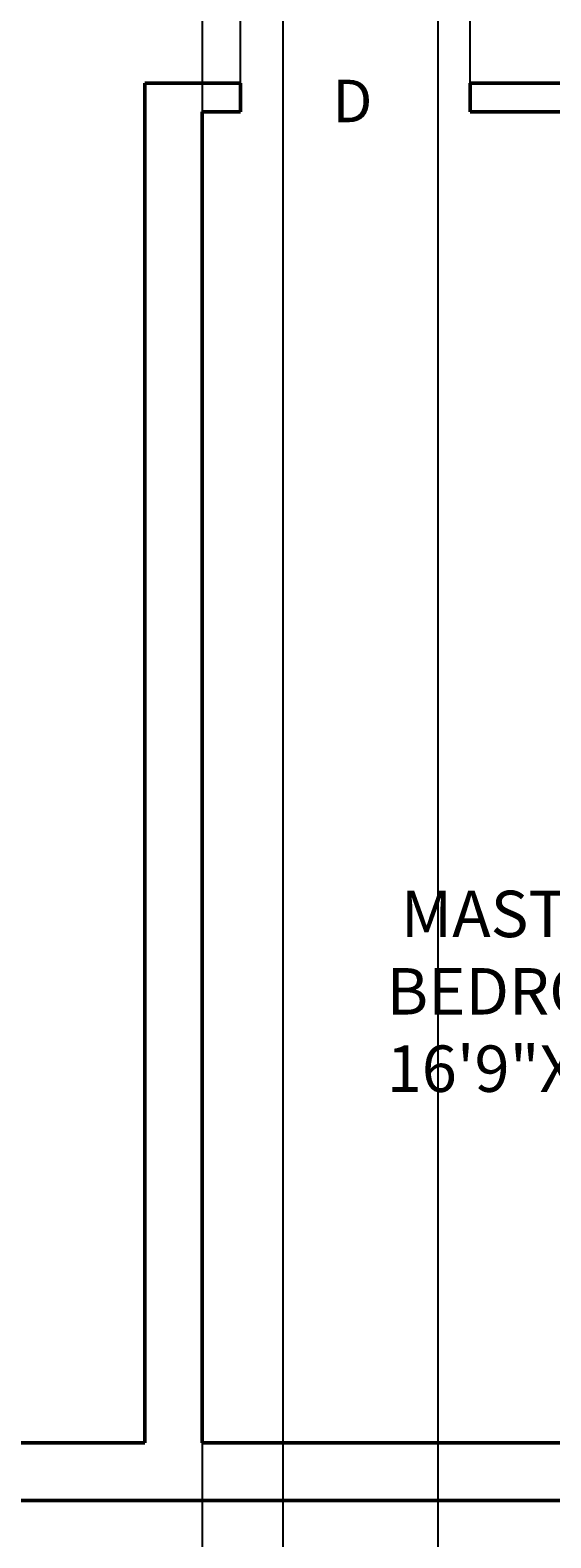
# Model space of a CAD drawing. Units: inches. Extents: x 338 to 1188, y -996 to 127.
# Tile 8 of 15: x 720 to 802, y -622 to -385. Entities that reach past the tile are written whole.
import ezdxf

# ---------------------------------------------------------------- set-up
doc = ezdxf.new("R2010")
doc.units = ezdxf.units.IN
doc.header["$MEASUREMENT"] = 0
for name, color, linetype, lineweight in [('A-ANNO-DIMS', 5, 'Continuous', 18), ('A-ANNO-TEXT', 7, 'Continuous', 18), ('A-AREA-IDEN', 8, 'Continuous', 18), ('wall', 1, 'Continuous', 50)]:
    doc.layers.add(name, color=color, linetype=linetype, lineweight=lineweight)
doc.styles.get("Standard").update_dxf_attribs({"font": 'arial.ttf'})
doc.dimstyles.get("Standard").update_dxf_attribs({"dimtxt": 0.18, "dimasz": 0.18, "dimexe": 0.18, "dimexo": 0.0625, "dimgap": 0.09, "dimtad": 0, "dimtih": 1, "dimtoh": 1, "dimdec": 1, "dimzin": 0, "dimdsep": 46, "dimlunit": 4, "dimtxsty": 'Standard', "dimcen": 0.09, "dimadec": 0, "dimazin": 0, "dimtfac": 1, "dimtdec": 1, "dimtofl": 0, "dimtmove": 0, "dimatfit": 3, "dimfxl": 1, "dimtolj": 1, "dimtzin": 0, "dimarcsym": 0})

# ---------------------------------------------------------------- blocks, each defined once
blk = doc.blocks.new('*D37')
at = {"layer": 'A-ANNO-DIMS', "color": 0, "lineweight": -2, "transparency": 16777216}
for p, q in [((752.96, -393.67), (752.96, 67.25)), ((753.14, 67.07), (770.63, 67.07)), ((788.78, 67.07), (771.29, 67.07)), ((788.96, -393.67), (788.96, 67.25))]:
    blk.add_line(p, q, dxfattribs=at)
at = {"layer": 'A-ANNO-DIMS', "color": 0, "transparency": 16777216}
for points in [[(753.14, 67.1), (753.14, 67.04), (752.96, 67.07)], [(788.78, 67.1), (788.78, 67.04), (788.96, 67.07)]]:
    blk.add_solid(points, dxfattribs=at)
at = {"layer": 'Defpoints', "color": 0, "transparency": 16777216}
for p in [(788.96, 67.07), (752.96, -393.73), (788.96, -393.73)]:
    blk.add_point(p, dxfattribs=at)
at = {"layer": 'A-ANNO-DIMS', "color": 0, "transparency": 16777216, "insert": (770.96, 67.07), "char_height": 0.18, "attachment_point": 5}
blk.add_mtext('\\A1;3\'-0"', dxfattribs=at)
blk = doc.blocks.new('*D42')
at = {"layer": 'A-ANNO-DIMS', "color": 0, "lineweight": -2, "transparency": 16777216}
for p, q in [((746.96, -54.8), (746.96, -968.86)), ((783.89, -54.8), (783.89, -968.86)), ((747.14, -968.68), (765.1, -968.68)), ((783.71, -968.68), (765.76, -968.68))]:
    blk.add_line(p, q, dxfattribs=at)
at = {"layer": 'A-ANNO-DIMS', "color": 0, "transparency": 16777216}
for points in [[(747.14, -968.65), (747.14, -968.71), (746.96, -968.68)], [(783.71, -968.65), (783.71, -968.71), (783.89, -968.68)]]:
    blk.add_solid(points, dxfattribs=at)
at = {"layer": 'Defpoints', "color": 0, "transparency": 16777216}
for p in [(746.96, -54.73), (783.89, -54.73), (783.89, -968.68)]:
    blk.add_point(p, dxfattribs=at)
at = {"layer": 'A-ANNO-DIMS', "color": 0, "transparency": 16777216, "insert": (765.43, -968.68), "char_height": 0.18, "attachment_point": 5}
blk.add_mtext('\\A1;3\'-1"', dxfattribs=at)
blk = doc.blocks.new('*D47')
at = {"layer": 'A-ANNO-DIMS', "color": 0, "lineweight": -2, "transparency": 16777216}
for p, q in [((759.67, -755.17), (759.67, 67.25)), ((759.85, 67.07), (867.68, 67.07)), ((976.28, 67.07), (868.46, 67.07)), ((976.46, -755.17), (976.46, 67.25))]:
    blk.add_line(p, q, dxfattribs=at)
at = {"layer": 'A-ANNO-DIMS', "color": 0, "transparency": 16777216}
for points in [[(759.85, 67.1), (759.85, 67.04), (759.67, 67.07)], [(976.28, 67.1), (976.28, 67.04), (976.46, 67.07)]]:
    blk.add_solid(points, dxfattribs=at)
at = {"layer": 'Defpoints', "color": 0, "transparency": 16777216}
for p in [(976.46, 67.07), (759.67, -755.23), (976.46, -755.23)]:
    blk.add_point(p, dxfattribs=at)
at = {"layer": 'A-ANNO-DIMS', "color": 0, "transparency": 16777216, "insert": (868.07, 67.07), "char_height": 0.18, "attachment_point": 5}
blk.add_mtext('\\A1;18\'-1"', dxfattribs=at)

msp = doc.modelspace()

# ---------------------------------------------------------------- linework, layer by layer
at = {"layer": 'wall'}
for p, q in [((737.96, -393.73), (737.96, -606.73)), ((752.96, -393.73), (737.96, -393.73)), ((752.96, -393.73), (752.96, -398.23)), ((947.96, -393.73), (788.96, -393.73)), ((788.96, -393.73), (788.96, -398.23)), ((746.96, -398.23), (746.96, -606.73)), ((752.96, -398.23), (746.96, -398.23)), ((811.46, -398.23), (788.96, -398.23)), ((737.96, -606.73), (660.96, -606.73)), ((947.96, -606.73), (746.96, -606.73)), ((956.96, -615.73), (660.96, -615.73))]:
    msp.add_line(p, q, dxfattribs=at)

# ---------------------------------------------------------------- texts
at = {"layer": 'A-ANNO-TEXT'}
msp.add_text('D', height=6.65, dxfattribs=at).set_placement((767.39, -399.83))
at = {"layer": 'A-AREA-IDEN', "insert": (775.86, -520.22), "char_height": 7.2703, "attachment_point": 1}
msp.add_mtext_dynamic_manual_height_columns(' MASTER   BEDROOM              16\'9"X11\'', width=58.3567, gutter_width=1, heights=[0], dxfattribs=at)

# ---------------------------------------------------------------- dimensions: what is measured, and where the dimension line sits
at = {"layer": 'A-ANNO-DIMS'}
for base, p1, p2, picture, middle in [((788.96, 67.07), (752.96, -393.73), (788.96, -393.73), '*D37', (770.96, 67.07)), ((976.46, 67.07), (759.67, -755.23), (976.46, -755.23), '*D47', (868.07, 67.07)), ((783.89, -968.68), (746.96, -54.73), (783.89, -54.73), '*D42', (765.43, -968.68))]:
    dim = msp.add_linear_dim(base=base, p1=p1, p2=p2, dimstyle='Standard', override={"dimdec": 1, "dimlfac": 1, "dimrnd": 0, "dimzin": 1, "dimdsep": 46, "dimlunit": 4, "dimfrac": 2}, dxfattribs=at)
    dim.commit()
    dim.dimension.update_dxf_attribs({"geometry": picture, "text_midpoint": middle})

doc.saveas('drawing.dxf')
